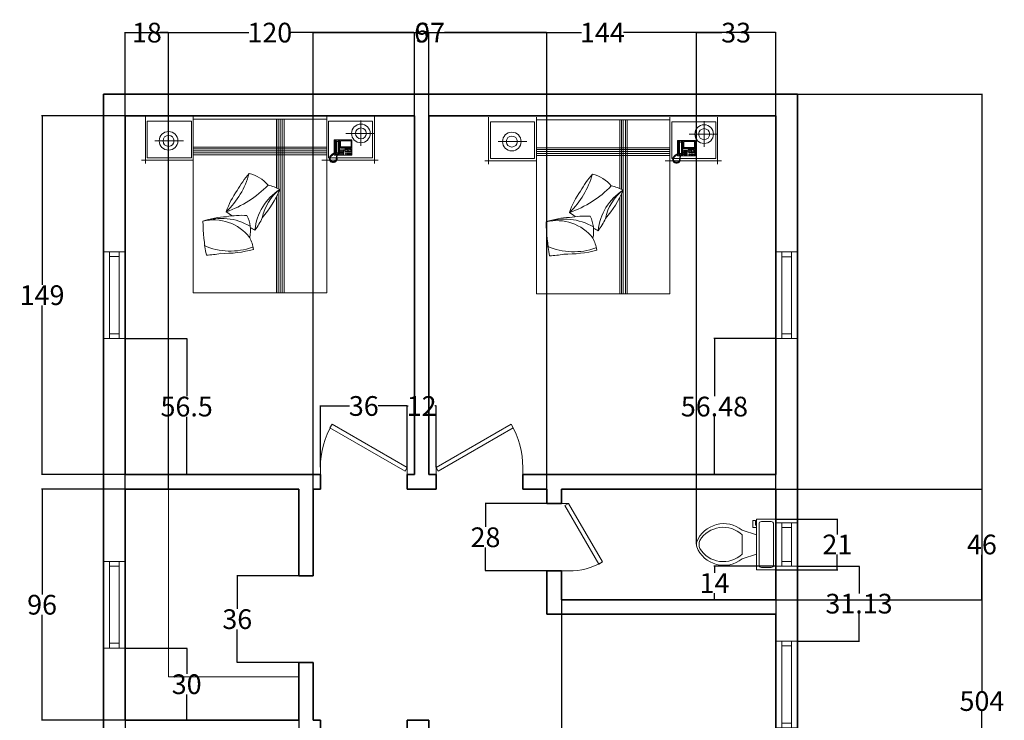
# Model space of a CAD drawing. Units: inches. Extents: x -254 to 1961, y 86 to 3025.
# Tile 3 of 6: x 117 to 525, y 408 to 699. Entities that reach past the tile are written whole.
import ezdxf

# ---------------------------------------------------------------- set-up
doc = ezdxf.new("R2010")
doc.units = ezdxf.units.IN
doc.header["$MEASUREMENT"] = 0
for name, color, linetype, lineweight in [('A-ANNO-DIMS', 2, 'Continuous', 18), ('A-FLOR-FIXT', 4, 'Continuous', 18), ('DOORS', 40, 'Continuous', 18), ('FURNITURE', 151, 'Continuous', 13), ('KITCHEN', 9, 'Continuous', 18), ('WALLS', 255, 'Continuous', 35), ('WINDOWS', 50, 'Continuous', 18)]:
    doc.layers.add(name, color=color, linetype=linetype, lineweight=lineweight)
doc.styles.get("Standard").update_dxf_attribs({"font": 'arial.ttf'})
doc.dimstyles.get("Standard").update_dxf_attribs({"dimtxt": 8.18, "dimasz": 0.18, "dimexe": 0.18, "dimexo": 0.0625, "dimgap": 0.09, "dimtad": 0, "dimtih": 1, "dimtoh": 1, "dimdec": 1, "dimzin": 0, "dimdsep": 46, "dimlunit": 3, "dimtxsty": 'Standard', "dimcen": 0.09, "dimadec": 0, "dimazin": 0, "dimtfac": 1, "dimtdec": 1, "dimtofl": 0, "dimtmove": 0, "dimatfit": 3, "dimfxl": 1, "dimtolj": 1, "dimtzin": 0, "dimarcsym": 0})

# ---------------------------------------------------------------- blocks, each defined once
blk = doc.blocks.new('*U5')
for p, q in [((0, 0), (0, -6)), ((36, 0), (36, -6))]:
    blk.add_line(p, q)
blk.add_lwpolyline([(0, 0), (31.18, 18), (32.05, 16.48), (0.87, -1.52)], close=True)
blk.add_arc((0, 0), 36, 0, 30)
blk = doc.blocks.new('*U4')
for p, q in [((0, 0), (0, -6)), ((-36, 0), (-36, -6))]:
    blk.add_line(p, q)
blk.add_lwpolyline([(0, 0), (-31.18, 18), (-32.05, 16.48), (-0.88, -1.52)], close=True)
blk.add_arc((0, 0), 36, 150, 180)
blk = doc.blocks.new('*U6')
for p, q in [((0, 0), (0, -6)), ((28, 0), (28, -6))]:
    blk.add_line(p, q)
blk.add_lwpolyline([(0, 0), (24.25, 14), (25.12, 12.48), (0.87, -1.52)], close=True)
blk.add_arc((0, 0), 28, 0, 30)
blk = doc.blocks.new('*U9')
for p, q in [((9.5, -6), (9.5, -2)), ((-8, -8.5), (-8, -8)), ((-7, -8), (-7, -9.5)), ((-4, -8), (-6, -14)), ((4, -8), (6, -14)), ((-10, -8.5), (-8, -8.5)), ((-10, -9.5), (-10, -8.5)), ((-7, -9.5), (-10, -9.5)), ((4, -14), (-4, -14))]:
    blk.add_line(p, q)
blk.add_lwpolyline([(10.5, -8), (10.5, 0), (-10.5, 0), (-10.5, -8)], close=True)
for points in [[(-9.5, -2), (-9.5, -6)], [(8.5, -1), (-8.5, -1)], [(-8.5, -7), (8.5, -7)]]:
    blk.add_lwpolyline(points)
for centre, radius, start, end in [((-8.62, -1.88), 0.884, 81.8699, 188.1301), ((8.62, -1.88), 0.884, 351.8699, 98.1301), ((-8.62, -6.12), 0.884, 171.8699, 278.1301), ((8.62, -6.12), 0.884, 261.8699, 8.1301), ((3.52, -21.58), 12.17, 141.4691, 247.9714), ((4.2, -21.82), 11.33, 136.3677, 238.9468), ((-3.52, -21.58), 12.17, 292.0284, 38.5307), ((-4.2, -21.82), 11.33, 301.053, 43.6321), ((0, -27.88), 4, 245.7318, 294.2682), ((0, -29), 4, 254.8605, 285.1395)]:
    blk.add_arc(centre, radius, start, end)
blk = doc.blocks.new('BED-DOUBLE-NIGHTSTANDS')
for p, q in [((1.58, 73.32), (1.58, 53.78)), ((20.68, 71.37), (2.35, 71.37)), ((2.35, 71.37), (2.35, 56.1)), ((20.68, 56.1), (20.68, 71.37)), ((21.4, 73.32), (21.4, 53.78)), ((76.84, 72.19), (21.4, 72.19)), ((21.4, 72.19), (21.4, 0)), ((55.98, 43.63), (55.98, 72.19)), ((56.73, 43.3), (56.73, 72.19)), ((57.47, 0), (57.47, 72.19)), ((58.37, 0), (58.37, 72.19)), ((59.13, 0), (59.13, 72.19)), ((76.84, 73.32), (76.84, 53.78)), ((76.84, 0), (76.84, 72.19)), ((77.56, 56.1), (77.56, 71.37)), ((77.56, 71.37), (95.89, 71.37)), ((91.03, 61.02), (91.03, 71.64)), ((95.89, 71.37), (95.89, 56.1)), ((96.61, 73.32), (96.61, 53.78)), ((96.71, 66.24), (84.84, 66.24)), ((5.54, 63.15), (17.4, 63.15)), ((79.99, 63.51), (80.08, 63.61)), ((79.99, 57.27), (79.99, 63.51)), ((80.08, 63.61), (87.23, 63.61)), ((80.58, 63.47), (80.35, 63.24)), ((80.35, 63.24), (80.35, 57.81)), ((80.49, 63.33), (80.44, 63.15)), ((80.85, 62.75), (80.44, 63.15)), ((80.44, 63.15), (80.44, 61.93)), ((80.44, 61.93), (80.54, 61.7)), ((80.67, 63.42), (80.49, 63.33)), ((80.54, 61.7), (80.67, 61.48)), ((81.94, 63.47), (80.58, 63.47)), ((81.76, 63.42), (80.67, 63.42)), ((80.9, 62.84), (80.67, 63.42)), ((80.67, 61.48), (80.72, 61.16)), ((80.9, 62.84), (80.85, 62.75)), ((80.85, 62.75), (80.85, 60.71)), ((81.53, 62.84), (80.9, 62.84)), ((81.76, 63.42), (81.53, 62.84)), ((81.58, 62.75), (81.53, 62.84)), ((81.98, 63.15), (81.58, 62.75)), ((81.58, 62.75), (81.58, 60.71)), ((81.71, 61.16), (81.76, 61.48)), ((81.94, 63.33), (81.76, 63.42)), ((81.76, 61.48), (81.89, 61.7)), ((81.89, 61.7), (81.98, 61.93)), ((82.12, 63.24), (81.94, 63.47)), ((81.98, 63.15), (81.94, 63.33)), ((81.98, 61.93), (81.98, 63.15)), ((82.12, 57.77), (82.12, 63.24)), ((82.53, 60.71), (82.53, 63.11)), ((82.53, 63.11), (87.05, 63.11)), ((87.05, 63.11), (87.05, 60.71)), ((87.23, 63.61), (87.32, 63.51)), ((87.32, 63.51), (87.32, 57.27)), ((21.4, 60.55), (76.84, 60.55)), ((21.4, 59.81), (76.84, 59.81)), ((21.4, 59.06), (76.84, 59.06)), ((21.4, 58.17), (76.84, 58.17)), ((21.4, 57.41), (76.84, 57.41)), ((79.19, 57.22), (78.6, 56.71)), ((78.72, 57.24), (78.93, 57.44)), ((78.77, 56.95), (78.72, 57.24)), ((78.93, 57.44), (79.18, 57.31)), ((79.08, 57.58), (79.2, 57.7)), ((79.18, 57.31), (79.08, 57.58)), ((79.56, 57.55), (79.19, 57.22)), ((79.2, 57.7), (79.31, 57.62)), ((79.25, 57.75), (79.33, 57.83)), ((79.31, 57.62), (79.25, 57.75)), ((79.33, 57.83), (79.5, 57.77)), ((79.56, 57.64), (79.47, 57.65)), ((79.47, 57.65), (79.56, 57.55)), ((79.5, 57.77), (79.59, 57.85)), ((79.61, 57.7), (79.56, 57.64)), ((79.59, 57.85), (79.72, 57.98)), ((79.79, 57.85), (79.61, 57.7)), ((79.72, 57.98), (79.99, 58.08)), ((79.99, 57.9), (79.79, 57.85)), ((80.08, 57.18), (79.99, 57.27)), ((80.35, 57.81), (80.58, 57.54)), ((80.54, 59.31), (80.44, 59.08)), ((80.44, 59.08), (80.44, 57.86)), ((80.44, 57.86), (80.85, 58.26)), ((80.49, 57.68), (80.44, 57.86)), ((80.67, 57.59), (80.49, 57.68)), ((80.67, 59.53), (80.54, 59.31)), ((80.58, 57.54), (81.11, 57.54)), ((80.72, 59.85), (80.67, 59.53)), ((80.67, 57.59), (80.9, 58.17)), ((81.11, 57.59), (80.67, 57.59)), ((80.72, 61.16), (80.72, 60.71)), ((80.72, 60.71), (80.72, 59.85)), ((80.85, 60.71), (80.85, 58.26)), ((80.85, 58.26), (80.9, 58.17)), ((80.9, 58.17), (81.53, 58.17)), ((81.03, 57.07), (81.1, 57.36)), ((81.1, 57.36), (81.12, 57.72)), ((81.12, 57.72), (81.26, 57.72)), ((81.25, 57.33), (81.14, 56.87)), ((81.26, 57.72), (81.25, 57.33)), ((81.76, 57.59), (81.26, 57.59)), ((81.26, 57.54), (81.89, 57.54)), ((81.58, 58.26), (81.53, 58.17)), ((81.53, 58.17), (81.76, 57.59)), ((81.58, 60.71), (81.58, 58.26)), ((81.98, 57.86), (81.58, 58.26)), ((81.71, 60.71), (81.71, 61.16)), ((81.71, 59.85), (81.71, 60.71)), ((82.12, 60.34), (81.71, 60.34)), ((81.76, 59.53), (81.71, 59.85)), ((81.89, 59.31), (81.76, 59.53)), ((81.76, 57.59), (81.94, 57.68)), ((81.98, 59.08), (81.89, 59.31)), ((81.89, 57.54), (82.12, 57.77)), ((81.94, 57.68), (81.98, 57.86)), ((81.98, 57.86), (81.98, 59.08)), ((87.05, 60.71), (82.53, 60.71)), ((82.53, 60.17), (82.53, 60.62)), ((82.53, 60.62), (86.87, 60.62)), ((86.87, 60.34), (82.53, 60.34)), ((86.87, 60.17), (82.53, 60.17)), ((82.89, 59.44), (82.53, 59.44)), ((82.53, 59.44), (82.53, 59.17)), ((82.53, 59.17), (82.89, 59.17)), ((82.89, 58.94), (82.53, 58.94)), ((82.53, 58.94), (82.53, 58.67)), ((82.53, 58.67), (82.89, 58.67)), ((82.53, 58.45), (82.53, 58.17)), ((82.89, 58.45), (82.53, 58.45)), ((82.53, 58.17), (82.89, 58.17)), ((82.53, 57.9), (82.53, 57.63)), ((82.89, 57.9), (82.53, 57.9)), ((82.53, 57.63), (82.89, 57.63)), ((82.89, 59.17), (82.89, 59.44)), ((82.89, 58.67), (82.89, 58.94)), ((82.89, 58.17), (82.89, 58.45)), ((82.89, 57.63), (82.89, 57.9)), ((83.07, 59.44), (83.07, 59.17)), ((83.43, 59.44), (83.07, 59.44)), ((83.07, 59.17), (83.43, 59.17)), ((83.43, 58.94), (83.07, 58.94)), ((83.07, 58.94), (83.07, 58.67)), ((83.07, 58.67), (83.43, 58.67)), ((83.07, 58.4), (83.07, 58.13)), ((83.43, 58.4), (83.07, 58.4)), ((83.07, 58.13), (83.43, 58.13)), ((83.43, 57.9), (83.07, 57.9)), ((83.07, 57.9), (83.07, 57.63)), ((83.07, 57.63), (83.43, 57.63)), ((83.43, 59.17), (83.43, 59.44)), ((83.43, 58.67), (83.43, 58.94)), ((83.43, 58.13), (83.43, 58.4)), ((83.43, 57.63), (83.43, 57.9)), ((83.97, 59.44), (83.61, 59.44)), ((83.61, 59.44), (83.61, 59.17)), ((83.61, 59.17), (83.97, 59.17)), ((83.97, 58.94), (83.61, 58.94)), ((83.61, 58.94), (83.61, 58.67)), ((83.61, 58.67), (83.97, 58.67)), ((83.97, 58.4), (83.61, 58.4)), ((83.61, 58.4), (83.61, 58.13)), ((83.61, 58.13), (83.97, 58.13)), ((83.97, 57.9), (83.61, 57.9)), ((83.61, 57.9), (83.61, 57.63)), ((83.61, 57.63), (83.97, 57.63)), ((83.97, 59.17), (83.97, 59.44)), ((83.97, 58.67), (83.97, 58.94)), ((83.97, 58.13), (83.97, 58.4)), ((83.97, 57.63), (83.97, 57.9)), ((84.38, 58.85), (84.38, 59.67)), ((84.38, 59.67), (87.05, 59.67)), ((87.05, 58.85), (84.38, 58.85)), ((84.73, 60.17), (84.56, 60.34)), ((84.65, 58.45), (84.65, 58.63)), ((84.65, 58.63), (85.11, 58.63)), ((85.11, 58.45), (84.65, 58.45)), ((85.11, 57.95), (84.65, 57.95)), ((84.65, 57.95), (84.65, 57.68)), ((84.65, 57.68), (85.11, 57.68)), ((84.7, 60.62), (84.7, 60.17)), ((84.83, 59.44), (84.83, 59.58)), ((84.83, 59.58), (84.97, 59.58)), ((84.97, 59.44), (84.83, 59.44)), ((84.83, 58.94), (84.83, 59.08)), ((84.83, 59.08), (84.97, 59.08)), ((84.97, 58.94), (84.83, 58.94)), ((84.97, 59.58), (84.97, 59.44)), ((84.97, 59.08), (84.97, 58.94)), ((85.06, 60.62), (85.06, 60.17)), ((85.11, 58.63), (85.11, 58.45)), ((85.11, 57.68), (85.11, 57.95)), ((86.04, 58.85), (85.23, 59.67)), ((85.29, 58.63), (85.74, 58.63)), ((85.29, 58.45), (85.29, 58.63)), ((85.74, 58.45), (85.29, 58.45)), ((85.29, 57.95), (85.29, 57.68)), ((85.74, 57.95), (85.29, 57.95)), ((85.29, 57.68), (85.74, 57.68)), ((85.42, 60.62), (85.42, 60.17)), ((85.65, 59.44), (85.65, 59.58)), ((85.65, 59.58), (85.79, 59.58)), ((85.79, 59.44), (85.65, 59.44)), ((85.65, 58.94), (85.65, 59.08)), ((85.65, 59.08), (85.79, 59.08)), ((85.79, 58.94), (85.65, 58.94)), ((85.74, 58.63), (85.74, 58.45)), ((85.74, 57.68), (85.74, 57.95)), ((85.79, 60.62), (85.79, 60.17)), ((85.79, 59.58), (85.79, 59.44)), ((85.79, 59.08), (85.79, 58.94)), ((85.92, 58.63), (86.37, 58.63)), ((85.92, 58.45), (85.92, 58.63)), ((86.37, 58.45), (85.92, 58.45)), ((85.92, 57.95), (85.92, 57.68)), ((86.37, 57.95), (85.92, 57.95)), ((85.92, 57.68), (86.37, 57.68)), ((86.15, 60.62), (86.15, 60.17)), ((86.37, 58.52), (86.27, 58.63)), ((86.37, 58.63), (86.37, 58.45)), ((86.37, 57.68), (86.37, 57.95)), ((86.46, 59.44), (86.46, 59.58)), ((86.46, 59.58), (86.6, 59.58)), ((86.6, 59.44), (86.46, 59.44)), ((86.46, 58.94), (86.46, 59.08)), ((86.46, 59.08), (86.6, 59.08)), ((86.6, 58.94), (86.46, 58.94)), ((86.51, 60.62), (86.51, 60.17)), ((86.55, 58.63), (87.01, 58.63)), ((86.55, 58.45), (86.55, 58.63)), ((87.01, 58.45), (86.55, 58.45)), ((86.55, 57.95), (86.55, 57.68)), ((87.01, 57.95), (86.55, 57.95)), ((86.55, 57.68), (87.01, 57.68)), ((86.6, 59.58), (86.6, 59.44)), ((86.6, 59.08), (86.6, 58.94)), ((86.87, 60.62), (86.87, 60.17)), ((87.01, 57.89), (86.95, 57.95)), ((87.01, 58.63), (87.01, 58.45)), ((87.01, 57.68), (87.01, 57.95)), ((87.05, 59.67), (87.05, 58.85)), ((87.32, 57.27), (87.23, 57.18)), ((0, 55.17), (21.4, 55.17)), ((2.35, 56.1), (20.68, 56.1)), ((98.24, 55.17), (74.88, 55.17)), ((95.89, 56.1), (77.56, 56.1)), ((77.91, 55.74), (77.96, 55.97)), ((78.19, 55.65), (77.91, 55.74)), ((77.96, 55.97), (78.2, 55.97)), ((77.96, 55.52), (78.19, 55.65)), ((77.99, 55.33), (77.96, 55.52)), ((78.28, 55.34), (77.99, 55.33)), ((78.01, 56.15), (78.07, 56.36)), ((78.2, 55.97), (78.01, 56.15)), ((78.06, 55.09), (78.28, 55.34)), ((78.13, 54.91), (78.06, 55.09)), ((78.07, 56.36), (78.37, 56.35)), ((78.1, 56.45), (78.18, 56.73)), ((78.37, 56.35), (78.1, 56.45)), ((78.4, 54.99), (78.13, 54.91)), ((78.18, 56.73), (78.46, 56.7)), ((78.38, 55.31), (78.24, 55.31)), ((78.27, 54.75), (78.4, 54.99)), ((78.39, 54.64), (78.27, 54.75)), ((78.59, 56.7), (78.29, 55.84)), ((78.29, 55.84), (78.41, 55.15)), ((78.39, 56.9), (78.56, 57.08)), ((78.46, 56.7), (78.39, 56.9)), ((78.64, 54.75), (78.39, 54.64)), ((78.41, 55.15), (78.82, 54.76)), ((78.53, 54.5), (78.64, 54.75)), ((78.68, 54.37), (78.53, 54.5)), ((78.56, 57.08), (78.77, 56.95)), ((78.87, 54.61), (78.68, 54.37)), ((78.82, 54.76), (79.35, 54.53)), ((78.84, 54.33), (78.87, 54.61)), ((78.99, 54.26), (78.84, 54.33)), ((79.2, 54.44), (78.99, 54.26)), ((79.21, 54.2), (79.2, 54.44)), ((79.38, 54.15), (79.21, 54.2)), ((79.35, 54.53), (79.9, 54.57)), ((79.49, 54.44), (79.38, 54.15)), ((79.55, 54.18), (79.49, 54.44)), ((79.71, 54.2), (79.55, 54.18)), ((79.82, 54.44), (79.71, 54.2)), ((79.93, 54.2), (79.82, 54.44)), ((79.9, 54.57), (80.38, 54.83)), ((80.13, 54.25), (79.93, 54.2)), ((81.06, 57.18), (80.08, 57.18)), ((80.32, 54.37), (80.1, 54.55)), ((80.1, 54.55), (80.13, 54.25)), ((80.49, 54.48), (80.32, 54.37)), ((80.38, 54.83), (80.73, 55.27)), ((80.67, 54.57), (80.46, 54.73)), ((80.46, 54.73), (80.49, 54.48)), ((80.8, 54.74), (80.67, 54.57)), ((80.95, 54.94), (80.68, 54.99)), ((80.68, 54.99), (80.8, 54.74)), ((80.73, 55.27), (80.78, 55.85)), ((80.74, 56.06), (80.9, 56.18)), ((80.78, 55.85), (80.74, 56.06)), ((81.11, 55.38), (80.81, 55.35)), ((80.81, 55.35), (81.07, 55.15)), ((81.13, 55.83), (80.87, 55.78)), ((80.87, 55.78), (81.12, 55.63)), ((80.9, 56.41), (80.92, 56.63)), ((80.9, 56.18), (80.9, 56.41)), ((80.92, 56.63), (81.03, 57.07)), ((81.07, 55.15), (80.95, 54.94)), ((81.04, 56.2), (81.01, 56.15)), ((81.01, 56.15), (81.12, 56.05)), ((81.14, 56.87), (81.03, 56.44)), ((81.03, 56.44), (81.04, 56.2)), ((81.12, 55.63), (81.11, 55.38)), ((81.12, 56.05), (81.13, 55.83)), ((87.23, 57.18), (81.22, 57.18)), ((56.73, 0), (56.73, 41.48)), ((55.98, 0), (55.98, 39.96)), ((21.4, 0), (76.84, 0))]:
    blk.add_line(p, q)
for centre, radius in [((91.03, 66.24), 3.87), ((11.21, 63.15), 3.87), ((11.21, 63.15), 2.29), ((91.03, 66.24), 2.29)]:
    blk.add_circle(centre, radius)
for centre, radius, start, end in [((11.42, 58.69), 34.44, 313.5807, 344.664), ((74.12, 23.89), 39.12, 138.9434, 151.5029), ((41.57, 35.76), 14.16, 39.5375, 77.5218), ((21.54, 74.27), 42.76, 288.5712, 316.3694), ((64.75, 23.92), 31.18, 143.3149, 161.6473), ((69.36, 24.04), 22.39, 122.3105, 174.6609), ((14.94, 61.05), 46.14, 319.6791, 336.9358), ((69.1, 27.6), 19.32, 127.3136, 169.3014), ((47.53, 23.64), 21.7, 62.9638, 76.7966), ((87.82, 103.02), 87.02, 232.7582, 234.7034), ((36.16, 0.49), 31.18, 91.7513, 110.0837), ((32.98, 6.89), 24.09, 59.8649, 108.19), ((29.97, 11.42), 18.9, 37.9983, 103.8151), ((112.46, 31.59), 87.02, 181.1946, 190.5116), ((41.96, -6.88), 39.12, 87.3798, 99.9393), ((31.02, 26.01), 14.16, 347.9738, 25.9582), ((23.83, 43.59), 29.07, 323.0649, 334.741), ((87.82, 103.02), 87.02, 240.6207, 242.0752), ((25.24, 13.81), 21.7, 11.4002, 25.233), ((36.91, 44.65), 27.26, 246.3586, 289.7064), ((26.13, 44.77), 29.07, 271.5012, 283.1774), ((34.28, 62.58), 46.14, 268.1155, 285.3722)]:
    blk.add_arc(centre, radius, start, end)
blk = doc.blocks.new('WIN-36IN')
for p, q in [((2.5, 35), (2.5, 2)), ((6.5, 35), (6.5, 2))]:
    blk.add_line(p, q)
for points in [[(0, 36), (9, 36), (9, 0), (0, 0)], [(2.5, 36), (6.5, 36), (6.5, 34), (2.5, 34)], [(2.5, 0), (6.5, 0), (6.5, 2), (2.5, 2)]]:
    blk.add_lwpolyline(points, close=True)
blk = doc.blocks.new('WIN-18IN')
for p, q in [((2.5, 16), (2.5, 2)), ((6.5, 16), (6.5, 2))]:
    blk.add_line(p, q)
for points in [[(0, 18), (9, 18), (9, 0), (0, 0)], [(2.5, 18), (6.5, 18), (6.5, 16), (2.5, 16)], [(2.5, 0), (6.5, 0), (6.5, 2), (2.5, 2)]]:
    blk.add_lwpolyline(points, close=True)
blk = doc.blocks.new('*D23')
at = {"layer": 'A-ANNO-DIMS', "color": 0, "lineweight": -2, "transparency": 16777216}
for p, q in [((439.44, 667.99), (516.06, 667.99)), ((515.88, 667.81), (515.88, 420.26)), ((515.88, 164.17), (515.88, 411.73)), ((439.44, 163.99), (516.06, 163.99))]:
    blk.add_line(p, q, dxfattribs=at)
at = {"layer": 'A-ANNO-DIMS', "color": 0, "transparency": 16777216}
for points in [[(515.85, 667.81), (515.91, 667.81), (515.88, 667.99)], [(515.85, 164.17), (515.91, 164.17), (515.88, 163.99)]]:
    blk.add_solid(points, dxfattribs=at)
at = {"layer": 'Defpoints', "color": 0, "transparency": 16777216}
for p in [(439.38, 667.99), (515.88, 667.99), (439.38, 163.99)]:
    blk.add_point(p, dxfattribs=at)
at = {"layer": 'A-ANNO-DIMS', "color": 0, "transparency": 16777216, "insert": (515.88, 415.99), "char_height": 8.18, "attachment_point": 5}
blk.add_mtext('\\A1;504', dxfattribs=at)
blk = doc.blocks.new('*D24')
at = {"layer": 'A-ANNO-DIMS', "color": 0, "lineweight": -2, "transparency": 16777216}
for p, q in [((160.38, 659.06), (160.38, 693.67)), ((160.56, 693.49), (211.65, 693.49)), ((280.2, 693.49), (229.11, 693.49)), ((280.38, 659.06), (280.38, 693.67))]:
    blk.add_line(p, q, dxfattribs=at)
at = {"layer": 'A-ANNO-DIMS', "color": 0, "transparency": 16777216}
for points in [[(160.56, 693.52), (160.56, 693.46), (160.38, 693.49)], [(280.2, 693.52), (280.2, 693.46), (280.38, 693.49)]]:
    blk.add_solid(points, dxfattribs=at)
at = {"layer": 'Defpoints', "color": 0, "transparency": 16777216}
for p in [(280.38, 693.49), (160.38, 658.99), (280.38, 658.99)]:
    blk.add_point(p, dxfattribs=at)
at = {"layer": 'A-ANNO-DIMS', "color": 0, "transparency": 16777216, "insert": (220.38, 693.49), "char_height": 8.18, "attachment_point": 5}
blk.add_mtext('\\A1;120', dxfattribs=at)
blk = doc.blocks.new('*D25')
at = {"layer": 'A-ANNO-DIMS', "color": 0, "lineweight": -2, "transparency": 16777216}
for p, q in [((286.38, 659.06), (286.38, 693.67)), ((286.56, 693.49), (349.66, 693.49)), ((430.2, 693.49), (367.11, 693.49)), ((430.38, 659.06), (430.38, 693.67))]:
    blk.add_line(p, q, dxfattribs=at)
at = {"layer": 'A-ANNO-DIMS', "color": 0, "transparency": 16777216}
for points in [[(286.56, 693.52), (286.56, 693.46), (286.38, 693.49)], [(430.2, 693.52), (430.2, 693.46), (430.38, 693.49)]]:
    blk.add_solid(points, dxfattribs=at)
at = {"layer": 'Defpoints', "color": 0, "transparency": 16777216}
for p in [(430.38, 693.49), (286.38, 658.99), (430.38, 658.99)]:
    blk.add_point(p, dxfattribs=at)
at = {"layer": 'A-ANNO-DIMS', "color": 0, "transparency": 16777216, "insert": (358.38, 693.49), "char_height": 8.18, "attachment_point": 5}
blk.add_mtext('\\A1;144', dxfattribs=at)
blk = doc.blocks.new('*D26')
at = {"layer": 'A-ANNO-DIMS', "color": 0, "lineweight": -2, "transparency": 16777216}
for p, q in [((280.201832, 693.494989), (280.021832, 693.494989)), ((280.381832, 659.057489), (280.381832, 693.674989)), ((286.381832, 659.057489), (286.381832, 693.674989)), ((286.561832, 693.494989), (286.741832, 693.494989))]:
    blk.add_line(p, q, dxfattribs=at)
at = {"layer": 'A-ANNO-DIMS', "color": 0, "transparency": 16777216}
for points in [[(280.201832, 693.524989), (280.201832, 693.464989), (280.381832, 693.494989)], [(286.561832, 693.524989), (286.561832, 693.464989), (286.381832, 693.494989)]]:
    blk.add_solid(points, dxfattribs=at)
at = {"layer": 'Defpoints', "color": 0, "transparency": 16777216}
for p in [(286.381832, 693.494989), (280.381832, 658.994989), (286.381832, 658.994989)]:
    blk.add_point(p, dxfattribs=at)
at = {"layer": 'A-ANNO-DIMS', "color": 0, "transparency": 16777216, "insert": (283.381832, 693.494989), "char_height": 8.18, "attachment_point": 5}
blk.add_mtext('\\A1;6', dxfattribs=at)
blk = doc.blocks.new('*D27')
at = {"layer": 'A-ANNO-DIMS', "color": 0, "lineweight": -2, "transparency": 16777216}
for p, q in [((241.38, 513.06), (241.38, 538.67)), ((241.56, 538.49), (253.44, 538.49)), ((277.2, 538.49), (265.33, 538.49)), ((277.38, 513.06), (277.38, 538.67))]:
    blk.add_line(p, q, dxfattribs=at)
at = {"layer": 'A-ANNO-DIMS', "color": 0, "transparency": 16777216}
for points in [[(241.56, 538.52), (241.56, 538.46), (241.38, 538.49)], [(277.2, 538.52), (277.2, 538.46), (277.38, 538.49)]]:
    blk.add_solid(points, dxfattribs=at)
at = {"layer": 'Defpoints', "color": 0, "transparency": 16777216}
for p in [(277.38, 538.49), (241.38, 512.99), (277.38, 512.99)]:
    blk.add_point(p, dxfattribs=at)
at = {"layer": 'A-ANNO-DIMS', "color": 0, "transparency": 16777216, "insert": (259.38, 538.49), "char_height": 8.18, "attachment_point": 5}
blk.add_mtext('\\A1;36', dxfattribs=at)
blk = doc.blocks.new('*D28')
at = {"layer": 'A-ANNO-DIMS', "color": 0, "lineweight": -2, "transparency": 16777216}
for p, q in [((277.38, 513.06), (277.38, 538.67)), ((277.56, 538.49), (277.86, 538.49)), ((289.2, 538.49), (288.9, 538.49)), ((289.38, 513.06), (289.38, 538.67))]:
    blk.add_line(p, q, dxfattribs=at)
at = {"layer": 'A-ANNO-DIMS', "color": 0, "transparency": 16777216}
for points in [[(277.56, 538.52), (277.56, 538.46), (277.38, 538.49)], [(289.2, 538.52), (289.2, 538.46), (289.38, 538.49)]]:
    blk.add_solid(points, dxfattribs=at)
at = {"layer": 'Defpoints', "color": 0, "transparency": 16777216}
for p in [(289.38, 538.49), (277.38, 512.99), (289.38, 512.99)]:
    blk.add_point(p, dxfattribs=at)
at = {"layer": 'A-ANNO-DIMS', "color": 0, "transparency": 16777216, "insert": (283.38, 538.49), "char_height": 8.18, "attachment_point": 5}
blk.add_mtext('\\A1;12', dxfattribs=at)
blk = doc.blocks.new('*D29')
at = {"layer": 'A-ANNO-DIMS', "color": 0, "lineweight": -2, "transparency": 16777216}
for p, q in [((160.32, 658.99), (125.7, 658.99)), ((125.88, 658.81), (125.88, 588.76)), ((125.88, 510.17), (125.88, 580.23)), ((160.32, 509.99), (125.7, 509.99))]:
    blk.add_line(p, q, dxfattribs=at)
at = {"layer": 'A-ANNO-DIMS', "color": 0, "transparency": 16777216}
for points in [[(125.85, 658.81), (125.91, 658.81), (125.88, 658.99)], [(125.85, 510.17), (125.91, 510.17), (125.88, 509.99)]]:
    blk.add_solid(points, dxfattribs=at)
at = {"layer": 'Defpoints', "color": 0, "transparency": 16777216}
for p in [(125.88, 658.99), (160.38, 658.99), (160.38, 509.99)]:
    blk.add_point(p, dxfattribs=at)
at = {"layer": 'A-ANNO-DIMS', "color": 0, "transparency": 16777216, "insert": (125.88, 584.49), "char_height": 8.18, "attachment_point": 5}
blk.add_mtext('\\A1;149', dxfattribs=at)
blk = doc.blocks.new('*D38')
at = {"layer": 'A-ANNO-DIMS', "color": 0, "lineweight": -2, "transparency": 16777216}
for p, q in [((160.44, 566.49), (186.06, 566.49)), ((185.88, 566.31), (185.88, 542.51)), ((185.88, 510.17), (185.88, 533.98)), ((160.44, 509.99), (186.06, 509.99))]:
    blk.add_line(p, q, dxfattribs=at)
at = {"layer": 'A-ANNO-DIMS', "color": 0, "transparency": 16777216}
for points in [[(185.85, 566.31), (185.91, 566.31), (185.88, 566.49)], [(185.85, 510.17), (185.91, 510.17), (185.88, 509.99)]]:
    blk.add_solid(points, dxfattribs=at)
at = {"layer": 'Defpoints', "color": 0, "transparency": 16777216}
for p in [(160.38, 566.49), (160.38, 509.99), (185.88, 509.99)]:
    blk.add_point(p, dxfattribs=at)
at = {"layer": 'A-ANNO-DIMS', "color": 0, "transparency": 16777216, "insert": (185.88, 538.24), "char_height": 8.18, "attachment_point": 5}
blk.add_mtext('\\A1;56.5', dxfattribs=at)
blk = doc.blocks.new('*D39')
at = {"layer": 'A-ANNO-DIMS', "color": 0, "lineweight": -2, "transparency": 16777216}
for p, q in [((430.32, 566.48), (404.7, 566.48)), ((404.88, 566.3), (404.88, 542.5)), ((404.88, 510.17), (404.88, 533.97)), ((430.32, 509.99), (404.7, 509.99))]:
    blk.add_line(p, q, dxfattribs=at)
at = {"layer": 'A-ANNO-DIMS', "color": 0, "transparency": 16777216}
for points in [[(404.85, 566.3), (404.91, 566.3), (404.88, 566.48)], [(404.85, 510.17), (404.91, 510.17), (404.88, 509.99)]]:
    blk.add_solid(points, dxfattribs=at)
at = {"layer": 'Defpoints', "color": 0, "transparency": 16777216}
for p in [(404.88, 566.48), (430.38, 566.48), (430.38, 509.99)]:
    blk.add_point(p, dxfattribs=at)
at = {"layer": 'A-ANNO-DIMS', "color": 0, "transparency": 16777216, "insert": (404.88, 538.24), "char_height": 8.18, "attachment_point": 5}
blk.add_mtext('\\A1;56.48', dxfattribs=at)
blk = doc.blocks.new('*D40')
at = {"layer": 'A-ANNO-DIMS', "color": 0, "lineweight": -2, "transparency": 16777216}
for p, q in [((439.44, 471.99), (465.06, 471.99)), ((464.88, 471.81), (464.88, 460.7)), ((464.88, 441.05), (464.88, 452.16)), ((439.44, 440.87), (465.06, 440.87))]:
    blk.add_line(p, q, dxfattribs=at)
at = {"layer": 'A-ANNO-DIMS', "color": 0, "transparency": 16777216}
for points in [[(464.85, 471.81), (464.91, 471.81), (464.88, 471.99)], [(464.85, 441.05), (464.91, 441.05), (464.88, 440.87)]]:
    blk.add_solid(points, dxfattribs=at)
at = {"layer": 'Defpoints', "color": 0, "transparency": 16777216}
for p in [(439.38, 471.99), (439.38, 440.87), (464.88, 440.87)]:
    blk.add_point(p, dxfattribs=at)
at = {"layer": 'A-ANNO-DIMS', "color": 0, "transparency": 16777216, "insert": (464.88, 456.43), "char_height": 8.18, "attachment_point": 5}
blk.add_mtext('\\A1;31.13', dxfattribs=at)
blk = doc.blocks.new('*D46')
at = {"layer": 'A-ANNO-DIMS', "color": 0, "lineweight": -2, "transparency": 16777216}
for p, q in [((160.38, 407.93), (160.38, 138.31)), ((232.38, 407.93), (232.38, 138.31)), ((160.56, 138.49), (190.51, 138.49)), ((232.2, 138.49), (202.26, 138.49))]:
    blk.add_line(p, q, dxfattribs=at)
at = {"layer": 'A-ANNO-DIMS', "color": 0, "transparency": 16777216}
for points in [[(160.56, 138.52), (160.56, 138.46), (160.38, 138.49)], [(232.2, 138.52), (232.2, 138.46), (232.38, 138.49)]]:
    blk.add_solid(points, dxfattribs=at)
at = {"layer": 'Defpoints', "color": 0, "transparency": 16777216}
for p in [(160.38, 407.99), (232.38, 407.99), (232.38, 138.49)]:
    blk.add_point(p, dxfattribs=at)
at = {"layer": 'A-ANNO-DIMS', "color": 0, "transparency": 16777216, "insert": (196.38, 138.49), "char_height": 8.18, "attachment_point": 5}
blk.add_mtext('\\A1;72', dxfattribs=at)
blk = doc.blocks.new('*D47')
at = {"layer": 'A-ANNO-DIMS', "color": 0, "lineweight": -2, "transparency": 16777216}
for p, q in [((160.32, 503.99), (125.7, 503.99)), ((125.88, 503.81), (125.88, 460.26)), ((125.88, 408.17), (125.88, 451.73)), ((160.32, 407.99), (125.7, 407.99))]:
    blk.add_line(p, q, dxfattribs=at)
at = {"layer": 'A-ANNO-DIMS', "color": 0, "transparency": 16777216}
for points in [[(125.85, 503.81), (125.91, 503.81), (125.88, 503.99)], [(125.85, 408.17), (125.91, 408.17), (125.88, 407.99)]]:
    blk.add_solid(points, dxfattribs=at)
at = {"layer": 'Defpoints', "color": 0, "transparency": 16777216}
for p in [(125.88, 503.99), (160.38, 503.99), (160.38, 407.99)]:
    blk.add_point(p, dxfattribs=at)
at = {"layer": 'A-ANNO-DIMS', "color": 0, "transparency": 16777216, "insert": (125.88, 455.99), "char_height": 8.18, "attachment_point": 5}
blk.add_mtext('\\A1;96', dxfattribs=at)
blk = doc.blocks.new('*D48')
at = {"layer": 'A-ANNO-DIMS', "color": 0, "lineweight": -2, "transparency": 16777216}
for p, q in [((341.38, 457.93), (341.38, 138.31)), ((430.38, 457.93), (430.38, 138.31)), ((341.56, 138.49), (379.92, 138.49)), ((430.2, 138.49), (391.84, 138.49))]:
    blk.add_line(p, q, dxfattribs=at)
at = {"layer": 'A-ANNO-DIMS', "color": 0, "transparency": 16777216}
for points in [[(341.56, 138.52), (341.56, 138.46), (341.38, 138.49)], [(430.2, 138.52), (430.2, 138.46), (430.38, 138.49)]]:
    blk.add_solid(points, dxfattribs=at)
at = {"layer": 'Defpoints', "color": 0, "transparency": 16777216}
for p in [(341.38, 457.99), (430.38, 457.99), (430.38, 138.49)]:
    blk.add_point(p, dxfattribs=at)
at = {"layer": 'A-ANNO-DIMS', "color": 0, "transparency": 16777216, "insert": (385.88, 138.49), "char_height": 8.18, "attachment_point": 5}
blk.add_mtext('\\A1;89', dxfattribs=at)
blk = doc.blocks.new('*D49')
at = {"layer": 'A-ANNO-DIMS', "color": 0, "lineweight": -2, "transparency": 16777216}
for p, q in [((430.44, 503.99), (516.06, 503.99)), ((515.88, 503.81), (515.88, 485.26)), ((515.88, 458.17), (515.88, 476.73)), ((430.44, 457.99), (516.06, 457.99))]:
    blk.add_line(p, q, dxfattribs=at)
at = {"layer": 'A-ANNO-DIMS', "color": 0, "transparency": 16777216}
for points in [[(515.85, 503.81), (515.91, 503.81), (515.88, 503.99)], [(515.85, 458.17), (515.91, 458.17), (515.88, 457.99)]]:
    blk.add_solid(points, dxfattribs=at)
at = {"layer": 'Defpoints', "color": 0, "transparency": 16777216}
for p in [(430.38, 503.99), (515.88, 503.99), (430.38, 457.99)]:
    blk.add_point(p, dxfattribs=at)
at = {"layer": 'A-ANNO-DIMS', "color": 0, "transparency": 16777216, "insert": (515.88, 480.99), "char_height": 8.18, "attachment_point": 5}
blk.add_mtext('\\A1;46', dxfattribs=at)
blk = doc.blocks.new('*D50')
at = {"layer": 'A-ANNO-DIMS', "color": 0, "lineweight": -2, "transparency": 16777216}
for p, q in [((238.38, 504.06), (238.38, 693.67)), ((238.56, 693.49), (280.93, 693.49)), ((335.2, 693.49), (292.83, 693.49)), ((335.38, 504.06), (335.38, 693.67))]:
    blk.add_line(p, q, dxfattribs=at)
at = {"layer": 'A-ANNO-DIMS', "color": 0, "transparency": 16777216}
for points in [[(238.56, 693.52), (238.56, 693.46), (238.38, 693.49)], [(335.2, 693.52), (335.2, 693.46), (335.38, 693.49)]]:
    blk.add_solid(points, dxfattribs=at)
at = {"layer": 'Defpoints', "color": 0, "transparency": 16777216}
for p in [(335.38, 693.49), (238.38, 503.99), (335.38, 503.99)]:
    blk.add_point(p, dxfattribs=at)
at = {"layer": 'A-ANNO-DIMS', "color": 0, "transparency": 16777216, "insert": (286.88, 693.49), "char_height": 8.18, "attachment_point": 5}
blk.add_mtext('\\A1;97', dxfattribs=at)
blk = doc.blocks.new('*D51')
at = {"layer": 'A-ANNO-DIMS', "color": 0, "lineweight": -2, "transparency": 16777216}
for p, q in [((335.32, 497.99), (309.7, 497.99)), ((309.88, 497.81), (309.88, 488.26)), ((309.88, 470.17), (309.88, 479.73)), ((335.32, 469.99), (309.7, 469.99))]:
    blk.add_line(p, q, dxfattribs=at)
at = {"layer": 'A-ANNO-DIMS', "color": 0, "transparency": 16777216}
for points in [[(309.85, 497.81), (309.91, 497.81), (309.88, 497.99)], [(309.85, 470.17), (309.91, 470.17), (309.88, 469.99)]]:
    blk.add_solid(points, dxfattribs=at)
at = {"layer": 'Defpoints', "color": 0, "transparency": 16777216}
for p in [(309.88, 497.99), (335.38, 497.99), (335.38, 469.99)]:
    blk.add_point(p, dxfattribs=at)
at = {"layer": 'A-ANNO-DIMS', "color": 0, "transparency": 16777216, "insert": (309.88, 483.99), "char_height": 8.18, "attachment_point": 5}
blk.add_mtext('\\A1;28', dxfattribs=at)
blk = doc.blocks.new('*D52')
at = {"layer": 'A-ANNO-DIMS', "color": 0, "lineweight": -2, "transparency": 16777216}
for p, q in [((232.32, 467.99), (206.7, 467.99)), ((206.88, 467.81), (206.88, 454.26)), ((206.88, 432.17), (206.88, 445.73)), ((232.32, 431.99), (206.7, 431.99))]:
    blk.add_line(p, q, dxfattribs=at)
at = {"layer": 'A-ANNO-DIMS', "color": 0, "transparency": 16777216}
for points in [[(206.85, 467.81), (206.91, 467.81), (206.88, 467.99)], [(206.85, 432.17), (206.91, 432.17), (206.88, 431.99)]]:
    blk.add_solid(points, dxfattribs=at)
at = {"layer": 'Defpoints', "color": 0, "transparency": 16777216}
for p in [(206.88, 467.99), (232.38, 467.99), (232.38, 431.99)]:
    blk.add_point(p, dxfattribs=at)
at = {"layer": 'A-ANNO-DIMS', "color": 0, "transparency": 16777216, "insert": (206.88, 449.99), "char_height": 8.18, "attachment_point": 5}
blk.add_mtext('\\A1;36', dxfattribs=at)
blk = doc.blocks.new('*D53')
at = {"layer": 'A-ANNO-DIMS', "color": 0, "lineweight": -2, "transparency": 16777216}
for p, q in [((160.44, 437.99), (186.06, 437.99)), ((185.88, 437.81), (185.88, 427.26)), ((185.88, 408.17), (185.88, 418.73)), ((160.44, 407.99), (186.06, 407.99))]:
    blk.add_line(p, q, dxfattribs=at)
at = {"layer": 'A-ANNO-DIMS', "color": 0, "transparency": 16777216}
for points in [[(185.85, 437.81), (185.91, 437.81), (185.88, 437.99)], [(185.85, 408.17), (185.91, 408.17), (185.88, 407.99)]]:
    blk.add_solid(points, dxfattribs=at)
at = {"layer": 'Defpoints', "color": 0, "transparency": 16777216}
for p in [(160.38, 437.99), (160.38, 407.99), (185.88, 407.99)]:
    blk.add_point(p, dxfattribs=at)
at = {"layer": 'A-ANNO-DIMS', "color": 0, "transparency": 16777216, "insert": (185.88, 422.99), "char_height": 8.18, "attachment_point": 5}
blk.add_mtext('\\A1;30', dxfattribs=at)
blk = doc.blocks.new('*D54')
at = {"layer": 'A-ANNO-DIMS', "color": 0, "lineweight": -2, "transparency": 16777216}
for p, q in [((430.32, 471.99), (404.7, 471.99)), ((404.88, 471.81), (404.88, 469.19)), ((430.32, 457.99), (404.7, 457.99)), ((404.88, 458.17), (404.88, 460.8))]:
    blk.add_line(p, q, dxfattribs=at)
at = {"layer": 'A-ANNO-DIMS', "color": 0, "transparency": 16777216}
for points in [[(404.85, 471.81), (404.91, 471.81), (404.88, 471.99)], [(404.85, 458.17), (404.91, 458.17), (404.88, 457.99)]]:
    blk.add_solid(points, dxfattribs=at)
at = {"layer": 'Defpoints', "color": 0, "transparency": 16777216}
for p in [(404.88, 471.99), (430.38, 471.99), (430.38, 457.99)]:
    blk.add_point(p, dxfattribs=at)
at = {"layer": 'A-ANNO-DIMS', "color": 0, "transparency": 16777216, "insert": (404.88, 464.99), "char_height": 8.18, "attachment_point": 5}
blk.add_mtext('\\A1;14', dxfattribs=at)
blk = doc.blocks.new('*D55')
at = {"layer": 'A-ANNO-DIMS', "color": 0, "lineweight": -2, "transparency": 16777216}
for p, q in [((160.38, 504.06), (160.38, 693.67)), ((160.56, 693.49), (163.81, 693.49)), ((178.2, 693.49), (174.95, 693.49)), ((178.38, 504.06), (178.38, 693.67))]:
    blk.add_line(p, q, dxfattribs=at)
at = {"layer": 'A-ANNO-DIMS', "color": 0, "transparency": 16777216}
for points in [[(160.56, 693.52), (160.56, 693.46), (160.38, 693.49)], [(178.2, 693.52), (178.2, 693.46), (178.38, 693.49)]]:
    blk.add_solid(points, dxfattribs=at)
at = {"layer": 'Defpoints', "color": 0, "transparency": 16777216}
for p in [(178.38, 693.49), (160.38, 503.99), (178.38, 503.99)]:
    blk.add_point(p, dxfattribs=at)
at = {"layer": 'A-ANNO-DIMS', "color": 0, "transparency": 16777216, "insert": (169.38, 693.49), "char_height": 8.18, "attachment_point": 5}
blk.add_mtext('\\A1;18', dxfattribs=at)
blk = doc.blocks.new('*D56')
at = {"layer": 'A-ANNO-DIMS', "color": 0, "lineweight": -2, "transparency": 16777216}
for p, q in [((430.44, 491.49), (456.06, 491.49)), ((455.88, 491.31), (455.88, 485.19)), ((455.88, 470.67), (455.88, 476.8)), ((430.44, 470.49), (456.06, 470.49))]:
    blk.add_line(p, q, dxfattribs=at)
at = {"layer": 'A-ANNO-DIMS', "color": 0, "transparency": 16777216}
for points in [[(455.85, 491.31), (455.91, 491.31), (455.88, 491.49)], [(455.85, 470.67), (455.91, 470.67), (455.88, 470.49)]]:
    blk.add_solid(points, dxfattribs=at)
at = {"layer": 'Defpoints', "color": 0, "transparency": 16777216}
for p in [(430.38, 491.49), (430.38, 470.49), (455.88, 470.49)]:
    blk.add_point(p, dxfattribs=at)
at = {"layer": 'A-ANNO-DIMS', "color": 0, "transparency": 16777216, "insert": (455.88, 480.99), "char_height": 8.18, "attachment_point": 5}
blk.add_mtext('\\A1;21', dxfattribs=at)
blk = doc.blocks.new('*D57')
at = {"layer": 'A-ANNO-DIMS', "color": 0, "lineweight": -2, "transparency": 16777216}
for p, q in [((397.38, 481.06), (397.38, 693.67)), ((397.56, 693.49), (407.94, 693.49)), ((430.2, 693.49), (419.83, 693.49)), ((430.38, 491.56), (430.38, 693.67))]:
    blk.add_line(p, q, dxfattribs=at)
at = {"layer": 'A-ANNO-DIMS', "color": 0, "transparency": 16777216}
for points in [[(397.56, 693.52), (397.56, 693.46), (397.38, 693.49)], [(430.2, 693.52), (430.2, 693.46), (430.38, 693.49)]]:
    blk.add_solid(points, dxfattribs=at)
at = {"layer": 'Defpoints', "color": 0, "transparency": 16777216}
for p in [(430.38, 693.49), (430.38, 491.49), (397.38, 480.99)]:
    blk.add_point(p, dxfattribs=at)
at = {"layer": 'A-ANNO-DIMS', "color": 0, "transparency": 16777216, "insert": (413.88, 693.49), "char_height": 8.18, "attachment_point": 5}
blk.add_mtext('\\A1;33', dxfattribs=at)

msp = doc.modelspace()

# ---------------------------------------------------------------- linework, layer by layer
at = {"layer": 'KITCHEN'}
for q in [(178.3818, 503.995), (232.3818, 425.995)]:
    msp.add_line((178.3818, 425.995), q, dxfattribs=at)
at = {"layer": 'WALLS'}
for p, q in [((151.3818, 163.995), (151.3818, 667.995)), ((151.3818, 667.995), (439.3818, 667.995)), ((439.3818, 163.995), (439.3818, 667.995)), ((160.3818, 658.995), (280.3818, 658.995)), ((160.3818, 509.995), (160.3818, 658.995)), ((280.3818, 509.995), (280.3818, 658.995)), ((286.3818, 509.995), (286.3818, 658.995)), ((286.3818, 658.995), (430.3818, 658.995)), ((430.3818, 509.995), (430.3818, 658.995)), ((160.3818, 509.995), (241.3818, 509.995)), ((241.3818, 503.995), (241.3818, 509.995)), ((277.3818, 509.995), (280.3818, 509.995)), ((277.3818, 503.995), (277.3818, 509.995)), ((286.3818, 509.995), (289.3818, 509.995)), ((289.3818, 503.995), (289.3818, 509.995)), ((325.3818, 503.995), (325.3818, 509.995)), ((325.3818, 509.995), (430.3818, 509.995)), ((160.3818, 503.995), (232.3818, 503.995)), ((160.3818, 407.995), (160.3818, 503.995)), ((232.3818, 467.995), (232.3818, 503.995)), ((238.3818, 503.995), (241.3818, 503.995)), ((238.3818, 467.995), (238.3818, 503.995)), ((277.3818, 503.995), (289.3818, 503.995)), ((325.3818, 503.995), (335.3818, 503.995)), ((335.3818, 497.995), (335.3818, 503.995)), ((341.3818, 497.995), (341.3818, 503.995)), ((341.3818, 503.995), (430.3818, 503.995)), ((430.3818, 457.995), (430.3818, 503.995)), ((335.3818, 497.995), (341.3818, 497.995)), ((335.3818, 451.995), (335.3818, 469.995)), ((335.3818, 469.995), (341.3818, 469.995)), ((341.3818, 457.995), (341.3818, 469.995)), ((232.3818, 467.995), (238.3818, 467.995)), ((341.3818, 457.995), (430.3818, 457.995)), ((335.3818, 451.995), (430.3818, 451.995)), ((430.3818, 280.995), (430.3818, 451.995)), ((232.3818, 407.995), (232.3818, 431.995)), ((232.3818, 431.995), (238.3818, 431.995)), ((238.3818, 407.995), (238.3818, 431.995)), ((160.3818, 407.995), (232.3818, 407.995)), ((238.3818, 407.995), (241.3818, 407.995)), ((241.3818, 401.995), (241.3818, 407.995)), ((277.3818, 401.995), (277.3818, 407.995)), ((277.3818, 407.995), (286.3818, 407.995)), ((286.3818, 280.995), (286.3818, 407.995))]:
    msp.add_line(p, q, dxfattribs=at)

# ---------------------------------------------------------------- block references
at = {"layer": 'A-FLOR-FIXT', "rotation": 270}
msp.add_blockref('*U9', (430.3818, 480.995), dxfattribs=at)
at = {"layer": 'DOORS'}
for name, p in [('*U4', (277.3818, 512.995)), ('*U5', (289.3818, 512.995))]:
    msp.add_blockref(name, p, dxfattribs=at)
at = {"layer": 'DOORS', "rotation": 270}
msp.add_blockref('*U6', (344.3818, 497.995), dxfattribs=at)
at = {"layer": 'FURNITURE'}
for p in [(167.155, 585.405), (309.6001, 585.1185)]:
    msp.add_blockref('BED-DOUBLE-NIGHTSTANDS', p, dxfattribs=at)
at = {"layer": 'WINDOWS'}
for name, p in [('WIN-36IN', (151.3819, 566.4949)), ('WIN-36IN', (430.3819, 566.4766)), ('WIN-18IN', (430.3817, 471.995)), ('WIN-36IN', (151.3819, 437.9949)), ('WIN-36IN', (430.3819, 404.8668))]:
    msp.add_blockref(name, p, dxfattribs=at)

# ---------------------------------------------------------------- texts
at = {"layer": 'FURNITURE', "flags": 9}
for tag, p, s in [('YSIZE', (207.4603, 614.1194), '806.5825'), ('XSIZE', (207.4603, 614.1193), '855.2549'), ('ZSIZE', (207.4603, 614.0885), '0.0000'), ('YSIZE', (349.9055, 613.8329), '806.5825'), ('XSIZE', (349.9055, 613.8328), '855.2549'), ('ZSIZE', (349.9055, 613.8019), '0.0000')]:
    msp.add_attdef(tag, p, s, height=0.0198, rotation=270, dxfattribs=at)

# ---------------------------------------------------------------- dimensions: what is measured, and where the dimension line sits
at = {"layer": 'A-ANNO-DIMS'}
for base, p1, p2, picture, middle in [((280.3818, 693.495), (160.3818, 658.995), (280.3818, 658.995), '*D24', (220.3818, 693.495)), ((178.3818, 693.495), (160.3818, 503.995), (178.3818, 503.995), '*D55', (169.3818, 693.495)), ((335.3818, 693.495), (238.3818, 503.995), (335.3818, 503.995), '*D50', (286.8818, 693.495)), ((286.3818, 693.495), (280.3818, 658.995), (286.3818, 658.995), '*D26', (283.3818, 693.495)), ((430.3818, 693.495), (286.3818, 658.995), (430.3818, 658.995), '*D25', (358.3818, 693.495)), ((430.3818, 693.495), (397.3819, 480.995), (430.3818, 491.495), '*D57', (413.8818, 693.495)), ((277.3818, 538.495), (241.3818, 512.995), (277.3818, 512.995), '*D27', (259.3818, 538.495)), ((289.3818, 538.495), (277.3818, 512.995), (289.3818, 512.995), '*D28', (283.3818, 538.495)), ((430.3818, 138.495), (341.3818, 457.995), (430.3818, 457.995), '*D48', (385.8818, 138.495)), ((232.3818, 138.495), (160.3818, 407.995), (232.3818, 407.995), '*D46', (196.3818, 138.495))]:
    dim = msp.add_linear_dim(base=base, p1=p1, p2=p2, dimstyle='Standard', override={"dimdec": 0, "dimlfac": 1, "dimrnd": 0, "dimzin": 0, "dimdsep": 46, "dimlunit": 2}, dxfattribs=at)
    dim.commit()
    dim.dimension.update_dxf_attribs({"geometry": picture, "text_midpoint": middle})
for base, p1, p2, angle, override, picture, middle in [((515.8818, 667.995), (439.3818, 163.995), (439.3818, 667.995), 90, {"dimdec": 0, "dimlfac": 1, "dimrnd": 0, "dimzin": 0, "dimdsep": 46, "dimlunit": 2}, '*D23', (515.8818, 415.995)), ((125.8818, 658.995), (160.3818, 509.995), (160.3818, 658.995), 90, {"dimdec": 0, "dimlfac": 1, "dimrnd": 0, "dimzin": 0, "dimdsep": 46, "dimlunit": 2}, '*D29', (125.8818, 584.495)), ((185.8818, 509.995), (160.3818, 566.495), (160.3818, 509.995), 270, {"dimdec": 1, "dimlfac": 1, "dimrnd": 0, "dimzin": 0, "dimdsep": 46, "dimlunit": 2}, '*D38', (185.8818, 538.245)), ((404.8818, 566.4767), (430.3818, 509.995), (430.3818, 566.4767), 90, {"dimdec": 2, "dimlfac": 1, "dimrnd": 0, "dimzin": 0, "dimdsep": 46, "dimlunit": 2}, '*D39', (404.8818, 538.2358)), ((125.8818, 503.995), (160.3818, 407.995), (160.3818, 503.995), 90, {"dimdec": 0, "dimlfac": 1, "dimrnd": 0, "dimzin": 0, "dimdsep": 46, "dimlunit": 2}, '*D47', (125.8818, 455.995)), ((515.8818, 503.995), (430.3818, 457.995), (430.3818, 503.995), 90, {"dimdec": 0, "dimlfac": 1, "dimrnd": 0, "dimzin": 0, "dimdsep": 46, "dimlunit": 2}, '*D49', (515.8818, 480.995)), ((309.8818, 497.995), (335.3818, 469.995), (335.3818, 497.995), 90, {"dimdec": 0, "dimlfac": 1, "dimrnd": 0, "dimzin": 0, "dimdsep": 46, "dimlunit": 2}, '*D51', (309.8818, 483.995)), ((455.8818, 470.495), (430.3818, 491.495), (430.3818, 470.495), 270, {"dimdec": 0, "dimlfac": 1, "dimrnd": 0, "dimzin": 0, "dimdsep": 46, "dimlunit": 2}, '*D56', (455.8818, 480.995)), ((404.8818, 471.995), (430.3818, 457.995), (430.3818, 471.995), 90, {"dimdec": 0, "dimlfac": 1, "dimrnd": 0, "dimzin": 0, "dimdsep": 46, "dimlunit": 2}, '*D54', (404.8818, 464.995)), ((464.8818, 440.8669), (439.3818, 471.995), (439.3818, 440.8669), 270, {"dimdec": 2, "dimlfac": 1, "dimrnd": 0, "dimzin": 0, "dimdsep": 46, "dimlunit": 2}, '*D40', (464.8818, 456.4309)), ((206.8818, 467.995), (232.3818, 431.995), (232.3818, 467.995), 90, {"dimdec": 0, "dimlfac": 1, "dimrnd": 0, "dimzin": 0, "dimdsep": 46, "dimlunit": 2}, '*D52', (206.8818, 449.995)), ((185.8818, 407.995), (160.3818, 437.995), (160.3818, 407.995), 270, {"dimdec": 0, "dimlfac": 1, "dimrnd": 0, "dimzin": 0, "dimdsep": 46, "dimlunit": 2}, '*D53', (185.8818, 422.995))]:
    dim = msp.add_linear_dim(base=base, p1=p1, p2=p2, angle=angle, dimstyle='Standard', override=override, dxfattribs=at)
    dim.commit()
    dim.dimension.update_dxf_attribs({"geometry": picture, "text_midpoint": middle})

doc.saveas('drawing.dxf')
